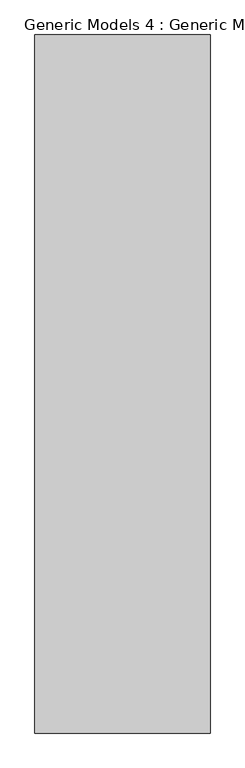
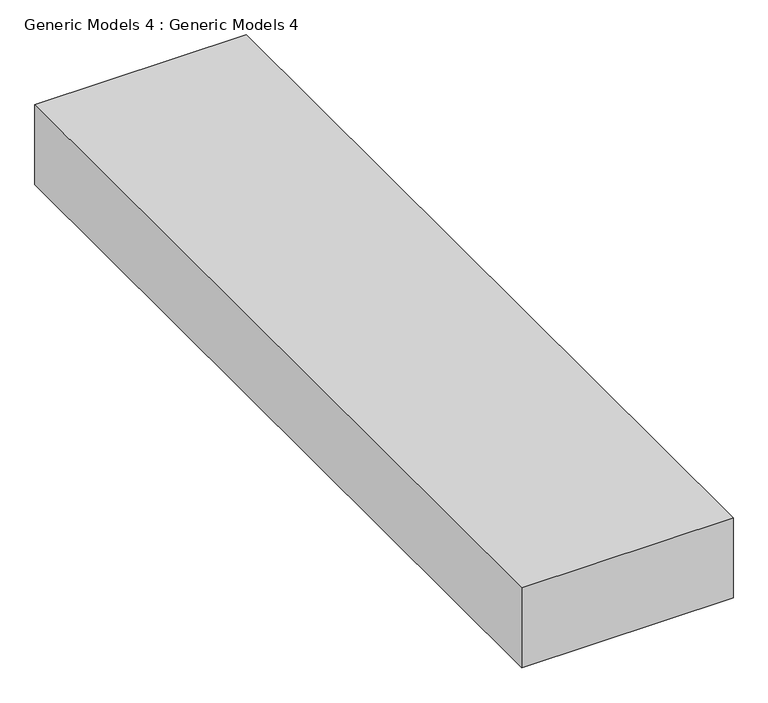
"""IFC4 building model written with IfcOpenShell, lengths in millimetres: proxy geometry, Generic Models 4 : Generic Models 4."""

from ifc_helpers import new_model, si_unit, frame, origin, place, context, project, spatial, polyline, outline, extrude, source, transform, mapped, element, save


def generic_models_4_generic_models_4_2a86e6bb(model_context):
    return source(origin(), model_context, "Body", "SweptSolid", [
        extrude(outline(polyline([(10520.2987508, -4408.7073314), (10520.2987508, -5932.7073314), (10137.9423568, -5932.7073314), (10137.9423568, -4408.7073314), (10520.2987508, -4408.7073314)])), frame((0.0, 0.0, 5572.0), z_axis=(0.0, 0.0, 1.0), x_axis=(1.0, 0.0, 0.0)), (0.0, 0.0, 1.0), 152.4),
    ])


if __name__ == "__main__":
    model = new_model("IFC4")
    model_context = context("Model", 3, world=origin())
    ifc_project = project(units=[si_unit("LENGTHUNIT", "METRE", prefix="MILLI")], contexts=[model_context])
    site = spatial("IfcSite", under=ifc_project)
    building = spatial("IfcBuilding", under=site)
    placement = place(None, origin())
    generic_models_4_generic_models_4_shape = generic_models_4_generic_models_4_2a86e6bb(model_context)
    element("IfcBuildingElementProxy", 1, Name="Generic Models 4 : Generic Models 4", ObjectType="Generic Models 4 : Generic Models 4", at=placement, inside=building, context=model_context, shape_type="MappedRepresentation", body=[
        mapped(generic_models_4_generic_models_4_shape, transform((0.0, 0.0, 0.0), x_axis=(1.0, 0.0, 0.0), y_axis=(0.0, 1.0, 0.0), z_axis=(0.0, 0.0, 1.0))),
    ])
    save(model, "model.ifc")

# Revit data of these elements
# Element 1 (IfcBuildingElementProxy, "Generic Models 4 : Generic Models 4")
#   Materials on its faces: "Clad - White"
# Materials
#   "Clad - White": class "Wood", colour RGB 242 242 238, transparency 0, Cost = 0
